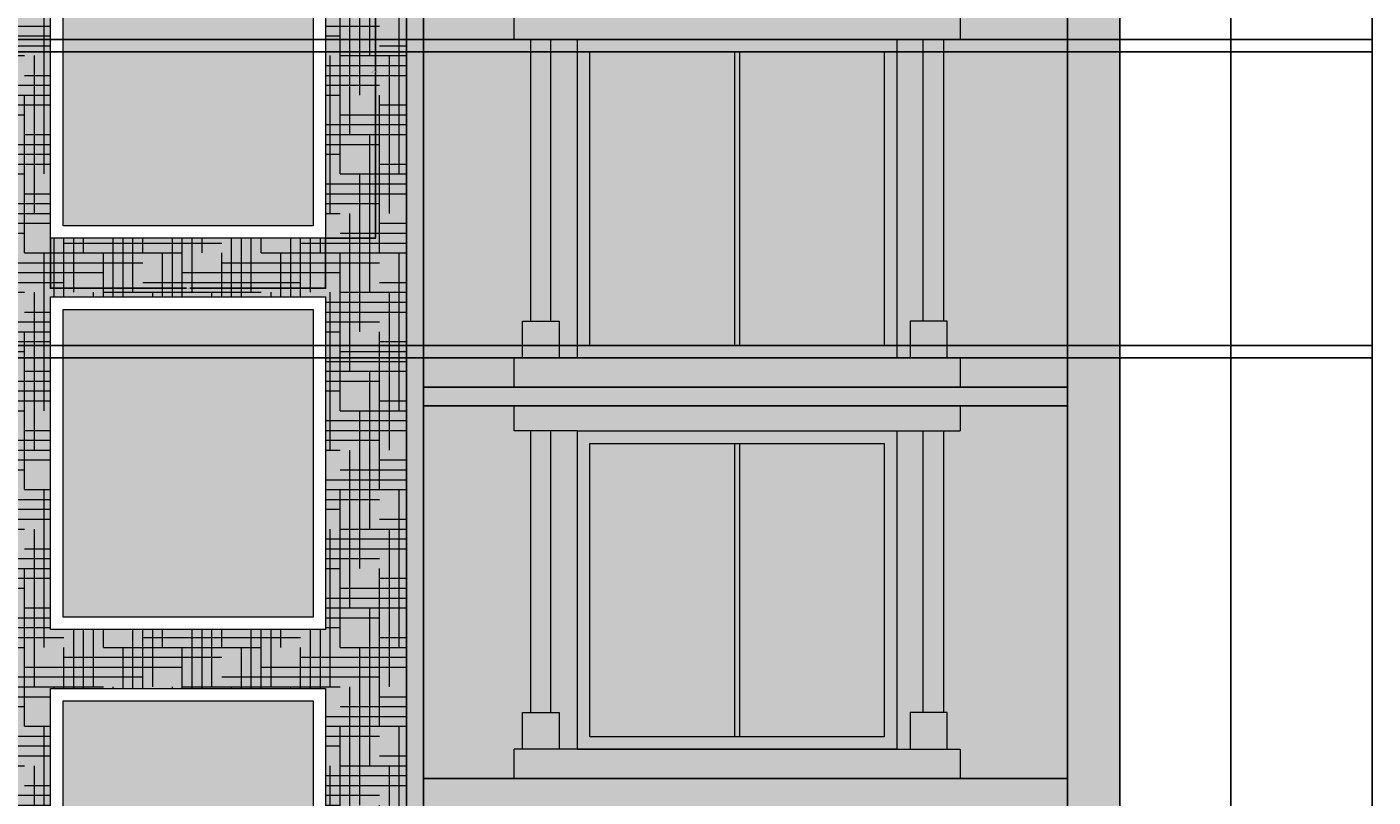
# Model space of a CAD drawing. Units: inches. Extents: x 3024 to 4744, y 1110 to 2100.
# Tile 26 of 29: x 3354 to 3787, y 1654 to 1902. Entities that reach past the tile are written whole.
import ezdxf

# ---------------------------------------------------------------- set-up
doc = ezdxf.new("R2010")
doc.units = ezdxf.units.IN
for name, color, linetype, lineweight in [('A-ANNO-DIMS', 2, 'Continuous', 18), ('A-ELEV', 7, 'Continuous', 25), ('A-ELEV-PATT', 252, 'Continuous', 13), ('A-GLAZ', 4, 'Continuous', 18)]:
    doc.layers.add(name, color=color, linetype=linetype, lineweight=lineweight)
doc.styles.get("Standard").update_dxf_attribs({"font": 'arial.ttf'})
doc.dimstyles.get("Standard").update_dxf_attribs({"dimtxt": 0.18, "dimasz": 0.18, "dimexe": 0.18, "dimexo": 0.0625, "dimgap": 0.09, "dimtad": 0, "dimtih": 1, "dimtoh": 1, "dimdec": 1, "dimzin": 0, "dimdsep": 46, "dimlunit": 3, "dimtxsty": 'Standard', "dimcen": 0.09, "dimadec": 0, "dimazin": 0, "dimtfac": 1, "dimtdec": 1, "dimtofl": 0, "dimtmove": 0, "dimatfit": 3, "dimfxl": 1, "dimtolj": 1, "dimtzin": 0, "dimarcsym": 0})

# ---------------------------------------------------------------- blocks, each defined once
blk = doc.blocks.new('WIN-BALCONY-A')
for p, q in [((3169.4, 1897.49), (3148.97, 1897.49)), ((3169.4, 1897.49), (3148.97, 1897.49)), ((3169.4, 1897.49), (3292.61, 1897.49)), ((3169.4, 1897.49), (3292.61, 1897.49)), ((3169.4, 1795.04), (3148.97, 1795.04)), ((3169.4, 1795.04), (3148.97, 1795.04)), ((3169.4, 1795.04), (3292.61, 1795.04)), ((3169.4, 1795.04), (3292.61, 1795.04))]:
    blk.add_line(p, q)
for points in [[(3148.97, 1897.49), (3148.97, 1905.61), (3292.61, 1905.61), (3292.61, 1897.49)], [(3148.97, 1897.49), (3148.97, 1905.61), (3292.61, 1905.61), (3292.61, 1897.49)], [(3292.61, 1795.04), (3292.61, 1785.61), (3148.97, 1785.61), (3148.97, 1795.04)], [(3292.61, 1795.04), (3292.61, 1785.61), (3148.97, 1785.61), (3148.97, 1795.04)]]:
    blk.add_lwpolyline(points)
for points in [[(3154.33, 1806.87), (3160.86, 1806.87), (3160.86, 1897.49), (3154.33, 1897.49)], [(3154.33, 1806.87), (3160.86, 1806.87), (3160.86, 1897.49), (3154.33, 1897.49)], [(3272.18, 1795.04), (3169.4, 1795.04), (3169.4, 1897.49), (3272.18, 1897.49)], [(3272.18, 1795.04), (3169.4, 1795.04), (3169.4, 1897.49), (3272.18, 1897.49)], [(3287.25, 1806.87), (3280.72, 1806.87), (3280.72, 1897.49), (3287.25, 1897.49)], [(3287.25, 1806.87), (3280.72, 1806.87), (3280.72, 1897.49), (3287.25, 1897.49)], [(3268.18, 1799.04), (3173.4, 1799.04), (3173.4, 1893.49), (3268.18, 1893.49)], [(3268.18, 1799.04), (3173.4, 1799.04), (3173.4, 1893.49), (3268.18, 1893.49)], [(3220.05, 1893.49), (3221.52, 1893.49), (3221.52, 1799.04), (3220.05, 1799.04)], [(3220.05, 1893.49), (3221.52, 1893.49), (3221.52, 1799.04), (3220.05, 1799.04)], [(3163.53, 1795.04), (3151.66, 1795.04), (3151.66, 1806.87), (3163.53, 1806.87)], [(3163.53, 1795.04), (3151.66, 1795.04), (3151.66, 1806.87), (3163.53, 1806.87)], [(3276.51, 1795.04), (3288.38, 1795.04), (3288.38, 1806.87), (3276.51, 1806.87)], [(3276.51, 1795.04), (3288.38, 1795.04), (3288.38, 1806.87), (3276.51, 1806.87)]]:
    blk.add_lwpolyline(points, close=True)
blk = doc.blocks.new('WIN-STONE-CENTRE')
for points in [[(3361.22, 1940.61), (3449.72, 1940.61), (3449.72, 1833.52), (3361.22, 1833.52)], [(3361.22, 1940.61), (3449.72, 1940.61), (3449.72, 1833.52), (3361.22, 1833.52)], [(3365.22, 1936.61), (3445.72, 1936.61), (3445.72, 1837.52), (3365.22, 1837.52)], [(3365.22, 1936.61), (3445.72, 1936.61), (3445.72, 1837.52), (3365.22, 1837.52)]]:
    blk.add_lwpolyline(points, close=True)
blk = doc.blocks.new('*D10')
at = {"layer": 'A-ANNO-DIMS', "color": 0, "lineweight": -2, "transparency": 16777216}
for p, q in [((3449.78, 1940.61), (3465.96, 1940.61)), ((3465.78, 1940.43), (3465.78, 1887.25)), ((3465.78, 1833.7), (3465.78, 1886.88)), ((3449.78, 1833.52), (3465.96, 1833.52))]:
    blk.add_line(p, q, dxfattribs=at)
at = {"layer": 'A-ANNO-DIMS', "color": 0, "transparency": 16777216}
for points in [[(3465.75, 1940.43), (3465.81, 1940.43), (3465.78, 1940.61)], [(3465.75, 1833.7), (3465.81, 1833.7), (3465.78, 1833.52)]]:
    blk.add_solid(points, dxfattribs=at)
at = {"layer": 'Defpoints', "color": 0, "transparency": 16777216}
for p in [(3449.72, 1940.61), (3465.78, 1940.61), (3449.72, 1833.52)]:
    blk.add_point(p, dxfattribs=at)
at = {"layer": 'A-ANNO-DIMS', "color": 0, "transparency": 16777216, "insert": (3465.78, 1887.07), "char_height": 0.18, "attachment_point": 5}
blk.add_mtext('\\A1;STONE WINDOW 107 TYP.', dxfattribs=at)
blk = doc.blocks.new('*D11')
at = {"layer": 'A-ANNO-DIMS', "color": 0, "lineweight": -2, "transparency": 16777216}
for p, q in [((3361.22, 1833.46), (3361.22, 1817.28)), ((3449.72, 1833.46), (3449.72, 1817.28)), ((3361.4, 1817.46), (3404.94, 1817.46)), ((3449.54, 1817.46), (3406, 1817.46))]:
    blk.add_line(p, q, dxfattribs=at)
at = {"layer": 'A-ANNO-DIMS', "color": 0, "transparency": 16777216}
for points in [[(3361.4, 1817.49), (3361.4, 1817.43), (3361.22, 1817.46)], [(3449.54, 1817.49), (3449.54, 1817.43), (3449.72, 1817.46)]]:
    blk.add_solid(points, dxfattribs=at)
at = {"layer": 'Defpoints', "color": 0, "transparency": 16777216}
for p in [(3361.22, 1833.52), (3449.72, 1833.52), (3449.72, 1817.46)]:
    blk.add_point(p, dxfattribs=at)
at = {"layer": 'A-ANNO-DIMS', "color": 0, "transparency": 16777216, "insert": (3405.47, 1817.46), "char_height": 0.18, "attachment_point": 5}
blk.add_mtext('\\A1;88 TYP.', dxfattribs=at)
blk = doc.blocks.new('*D64')
at = {"layer": 'A-ANNO-DIMS', "color": 0, "lineweight": -2, "transparency": 16777216}
for p, q in [((3069.79, 1241.5), (3069.79, 2100.44)), ((3069.97, 2100.26), (3405.08, 2100.26)), ((3740.97, 2100.26), (3405.87, 2100.26)), ((3741.15, 1241.5), (3741.15, 2100.44))]:
    blk.add_line(p, q, dxfattribs=at)
at = {"layer": 'A-ANNO-DIMS', "color": 0, "transparency": 16777216}
for points in [[(3069.97, 2100.29), (3069.97, 2100.23), (3069.79, 2100.26)], [(3740.97, 2100.29), (3740.97, 2100.23), (3741.15, 2100.26)]]:
    blk.add_solid(points, dxfattribs=at)
at = {"layer": 'Defpoints', "color": 0, "transparency": 16777216}
for p in [(3741.15, 2100.26), (3069.79, 1241.43), (3741.15, 1241.43)]:
    blk.add_point(p, dxfattribs=at)
at = {"layer": 'A-ANNO-DIMS', "color": 0, "transparency": 16777216, "insert": (3405.47, 2100.26), "char_height": 0.18, "attachment_point": 5}
blk.add_mtext('\\A1;671.4', dxfattribs=at)
blk = doc.blocks.new('*D75')
at = {"layer": 'A-ANNO-DIMS', "color": 0, "lineweight": -2, "transparency": 16777216}
for p, q in [((3491.89, 2054.76), (3786.83, 2054.76)), ((3786.65, 2054.58), (3786.65, 1605.37)), ((3786.65, 1155.79), (3786.65, 1605)), ((3741.21, 1155.61), (3786.83, 1155.61))]:
    blk.add_line(p, q, dxfattribs=at)
at = {"layer": 'A-ANNO-DIMS', "color": 0, "transparency": 16777216}
for points in [[(3786.62, 2054.58), (3786.68, 2054.58), (3786.65, 2054.76)], [(3786.62, 1155.79), (3786.68, 1155.79), (3786.65, 1155.61)]]:
    blk.add_solid(points, dxfattribs=at)
at = {"layer": 'Defpoints', "color": 0, "transparency": 16777216}
for p in [(3491.83, 2054.76), (3786.65, 2054.76), (3741.15, 1155.61)]:
    blk.add_point(p, dxfattribs=at)
at = {"layer": 'A-ANNO-DIMS', "color": 0, "transparency": 16777216, "insert": (3786.65, 1605.18), "char_height": 0.18, "attachment_point": 5}
blk.add_mtext('\\A1;899.1', dxfattribs=at)
blk = doc.blocks.new('*D100')
at = {"layer": 'A-ANNO-DIMS', "color": 0, "lineweight": -2, "transparency": 16777216}
for p, q in [((3268.24, 1799.04), (3786.83, 1799.04)), ((3786.65, 1798.86), (3786.65, 1797.23)), ((3272.24, 1795.04), (3786.83, 1795.04)), ((3786.65, 1795.22), (3786.65, 1796.86))]:
    blk.add_line(p, q, dxfattribs=at)
at = {"layer": 'A-ANNO-DIMS', "color": 0, "transparency": 16777216}
for points in [[(3786.62, 1798.86), (3786.68, 1798.86), (3786.65, 1799.04)], [(3786.62, 1795.22), (3786.68, 1795.22), (3786.65, 1795.04)]]:
    blk.add_solid(points, dxfattribs=at)
at = {"layer": 'Defpoints', "color": 0, "transparency": 16777216}
for p in [(3268.18, 1799.04), (3786.65, 1799.04), (3272.18, 1795.04)]:
    blk.add_point(p, dxfattribs=at)
at = {"layer": 'A-ANNO-DIMS', "color": 0, "transparency": 16777216, "insert": (3786.65, 1797.04), "char_height": 0.18, "attachment_point": 5}
blk.add_mtext('\\A1;4.00', dxfattribs=at)
blk = doc.blocks.new('*D101')
at = {"layer": 'A-ANNO-DIMS', "color": 0, "lineweight": -2, "transparency": 16777216}
for p, q in [((3268.24, 1893.49), (3786.83, 1893.49)), ((3786.65, 1893.31), (3786.65, 1846.45)), ((3786.65, 1799.22), (3786.65, 1846.08)), ((3268.24, 1799.04), (3786.83, 1799.04))]:
    blk.add_line(p, q, dxfattribs=at)
at = {"layer": 'A-ANNO-DIMS', "color": 0, "transparency": 16777216}
for points in [[(3786.62, 1893.31), (3786.68, 1893.31), (3786.65, 1893.49)], [(3786.62, 1799.22), (3786.68, 1799.22), (3786.65, 1799.04)]]:
    blk.add_solid(points, dxfattribs=at)
at = {"layer": 'Defpoints', "color": 0, "transparency": 16777216}
for p in [(3268.18, 1893.49), (3786.65, 1893.49), (3268.18, 1799.04)]:
    blk.add_point(p, dxfattribs=at)
at = {"layer": 'A-ANNO-DIMS', "color": 0, "transparency": 16777216, "insert": (3786.65, 1846.27), "char_height": 0.18, "attachment_point": 5}
blk.add_mtext('\\A1;94.44', dxfattribs=at)
blk = doc.blocks.new('*D102')
at = {"layer": 'A-ANNO-DIMS', "color": 0, "lineweight": -2, "transparency": 16777216}
for p, q in [((3272.24, 1897.49), (3786.83, 1897.49)), ((3786.65, 1897.31), (3786.65, 1895.67)), ((3786.65, 1893.67), (3786.65, 1895.31)), ((3268.24, 1893.49), (3786.83, 1893.49))]:
    blk.add_line(p, q, dxfattribs=at)
at = {"layer": 'A-ANNO-DIMS', "color": 0, "transparency": 16777216}
for points in [[(3786.62, 1897.31), (3786.68, 1897.31), (3786.65, 1897.49)], [(3786.62, 1893.67), (3786.68, 1893.67), (3786.65, 1893.49)]]:
    blk.add_solid(points, dxfattribs=at)
at = {"layer": 'Defpoints', "color": 0, "transparency": 16777216}
for p in [(3272.18, 1897.49), (3786.65, 1897.49), (3268.18, 1893.49)]:
    blk.add_point(p, dxfattribs=at)
at = {"layer": 'A-ANNO-DIMS', "color": 0, "transparency": 16777216, "insert": (3786.65, 1895.49), "char_height": 0.18, "attachment_point": 5}
blk.add_mtext('\\A1;4.00', dxfattribs=at)

msp = doc.modelspace()

# ---------------------------------------------------------------- hatches: boundary and pattern name
at = {"layer": 'A-ELEV-PATT'}
h = msp.add_hatch(color=256, dxfattribs=at)
h.dxf.hatch_style = 1
h.paths.add_polyline_path([(3491.8271, 2054.7584), (3320.5658, 2054.7584), (3320.5658, 2043.5286), (3491.8271, 2043.5286)])
h.paths.add_polyline_path([(3292.6051, 1905.6112), (3148.9694, 1905.6112), (3148.9694, 1897.4879), (3169.3964, 1897.4879), (3292.6051, 1897.4879)])
h.paths.add_polyline_path([(3292.6051, 1795.0431), (3169.3964, 1795.0431), (3148.9694, 1795.0431), (3148.9694, 1785.6112), (3292.6051, 1785.6112)])
h.paths.add_polyline_path([(3292.6051, 1779.6112), (3148.9694, 1779.6112), (3148.9694, 1771.4879), (3169.3964, 1771.4879), (3292.6051, 1771.4879)])
h.paths.add_polyline_path([(3292.6051, 1669.0431), (3169.3964, 1669.0431), (3148.9694, 1669.0431), (3148.9694, 1659.6112), (3292.6051, 1659.6112)])
h.paths.add_polyline_path([(3292.6051, 1653.6112), (3148.9694, 1653.6112), (3148.9694, 1645.4879), (3169.3964, 1645.4879), (3292.6051, 1645.4879)])
h.paths.add_polyline_path([(3292.6051, 1543.0431), (3169.3964, 1543.0431), (3148.9694, 1543.0431), (3148.9694, 1533.6112), (3292.6051, 1533.6112)])
h.paths.add_polyline_path([(3292.6051, 1527.6112), (3148.9694, 1527.6112), (3148.9694, 1519.4879), (3169.3964, 1519.4879), (3292.6051, 1519.4879)])
h.paths.add_polyline_path([(3292.6051, 1401.6112), (3148.9694, 1401.6112), (3148.9694, 1393.4879), (3169.3964, 1393.4879), (3292.6051, 1393.4879)])
h.paths.add_polyline_path([(3292.6051, 1417.0431), (3169.3964, 1417.0431), (3148.9694, 1417.0431), (3148.9694, 1407.6112), (3292.6051, 1407.6112)])
h.paths.add_polyline_path([(3292.6051, 1291.0431), (3169.3964, 1291.0431), (3148.9694, 1291.0431), (3148.9694, 1281.6112), (3292.6051, 1281.6112)])
h.paths.add_polyline_path([(3654.037, 1165.0431), (3530.8283, 1165.0431), (3510.4013, 1165.0431), (3510.4013, 1155.6112), (3654.037, 1155.6112)])
h.paths.add_polyline_path([(3654.037, 1275.6112), (3510.4013, 1275.6112), (3510.4013, 1267.4879), (3530.8283, 1267.4879), (3654.037, 1267.4879)])
h.paths.add_polyline_path([(3654.037, 1291.0431), (3530.8283, 1291.0431), (3510.4013, 1291.0431), (3510.4013, 1281.6112), (3654.037, 1281.6112)])
h.paths.add_polyline_path([(3654.037, 1417.0431), (3530.8283, 1417.0431), (3510.4013, 1417.0431), (3510.4013, 1407.6112), (3654.037, 1407.6112)])
h.paths.add_polyline_path([(3654.037, 1401.6112), (3510.4013, 1401.6112), (3510.4013, 1393.4879), (3530.8283, 1393.4879), (3654.037, 1393.4879)])
h.paths.add_polyline_path([(3654.037, 1543.0431), (3530.8283, 1543.0431), (3510.4013, 1543.0431), (3510.4013, 1533.6112), (3654.037, 1533.6112)])
h.paths.add_polyline_path([(3654.037, 1527.6112), (3510.4013, 1527.6112), (3510.4013, 1519.4879), (3530.8283, 1519.4879), (3654.037, 1519.4879)])
h.paths.add_polyline_path([(3654.037, 1653.6112), (3510.4013, 1653.6112), (3510.4013, 1645.4879), (3530.8283, 1645.4879), (3654.037, 1645.4879)])
h.paths.add_polyline_path([(3654.037, 1669.0431), (3530.8283, 1669.0431), (3510.4013, 1669.0431), (3510.4013, 1659.6112), (3654.037, 1659.6112)])
h.paths.add_polyline_path([(3654.037, 1779.6112), (3510.4013, 1779.6112), (3510.4013, 1771.4879), (3530.8283, 1771.4879), (3654.037, 1771.4879)])
h.paths.add_polyline_path([(3654.037, 1795.0431), (3530.8283, 1795.0431), (3510.4013, 1795.0431), (3510.4013, 1785.6112), (3654.037, 1785.6112)])
h.paths.add_polyline_path([(3654.037, 1905.6112), (3510.4013, 1905.6112), (3510.4013, 1897.4879), (3530.8283, 1897.4879), (3654.037, 1897.4879)])
h = msp.add_hatch(color=256, dxfattribs=at)
h.dxf.hatch_style = 1
h.paths.add_polyline_path([(3335.1044, 2043.5286), (3329.7033, 2043.5286), (3329.7033, 1155.6112), (3335.1044, 1155.6112)])
h.paths.add_polyline_path([(3481.2411, 2043.5286), (3335.1044, 2043.5286), (3335.1044, 1155.6112), (3481.2411, 1155.6112)])
h.paths.add_polyline_path([(3449.7202, 1329.5246), (3361.2242, 1329.5246), (3361.2242, 1436.6064), (3449.7202, 1436.6064)], flags=16)
h.paths.add_polyline_path([(3445.7202, 1333.5246), (3365.2242, 1333.5246), (3365.2242, 1432.6064), (3445.7202, 1432.6064)], flags=0)
h.paths.add_polyline_path([(3449.7202, 1455.5246), (3361.2242, 1455.5246), (3361.2242, 1562.6064), (3449.7202, 1562.6064)], flags=16)
h.paths.add_polyline_path([(3445.7202, 1459.5246), (3365.2242, 1459.5246), (3365.2242, 1558.6064), (3445.7202, 1558.6064)], flags=0)
h.paths.add_polyline_path([(3449.7202, 1581.5246), (3361.2242, 1581.5246), (3361.2242, 1688.6064), (3449.7202, 1688.6064)], flags=16)
h.paths.add_polyline_path([(3445.7202, 1585.5246), (3365.2242, 1585.5246), (3365.2242, 1684.6064), (3445.7202, 1684.6064)], flags=0)
h.paths.add_polyline_path([(3449.7202, 1707.5246), (3361.2242, 1707.5246), (3361.2242, 1814.6064), (3449.7202, 1814.6064)], flags=16)
h.paths.add_polyline_path([(3445.7202, 1711.5246), (3365.2242, 1711.5246), (3365.2242, 1810.6064), (3445.7202, 1810.6064)], flags=0)
h.paths.add_polyline_path([(3449.7202, 1833.5246), (3361.2242, 1833.5246), (3361.2242, 1940.6064), (3449.7202, 1940.6064)], flags=16)
h.paths.add_polyline_path([(3445.7202, 1837.5246), (3365.2242, 1837.5246), (3365.2242, 1936.6064), (3445.7202, 1936.6064)], flags=0)
h = msp.add_hatch(color=256, dxfattribs=at)
h.dxf.hatch_style = 1
h.paths.add_polyline_path([(3475.84, 2043.5286), (3335.1044, 2043.5286), (3335.1044, 1155.6112), (3475.84, 1155.6112)])
h.paths.add_polyline_path([(3449.7202, 1940.6064), (3449.7202, 1833.5246), (3361.2242, 1833.5246), (3361.2242, 1940.6064)], flags=16)
h.paths.add_polyline_path([(3445.7202, 1936.6064), (3445.7202, 1837.5246), (3365.2242, 1837.5246), (3365.2242, 1936.6064)], flags=0)
h.paths.add_polyline_path([(3449.7202, 1814.6064), (3449.7202, 1707.5246), (3361.2242, 1707.5246), (3361.2242, 1814.6064)], flags=16)
h.paths.add_polyline_path([(3445.7202, 1810.6064), (3445.7202, 1711.5246), (3365.2242, 1711.5246), (3365.2242, 1810.6064)], flags=0)
h.paths.add_polyline_path([(3449.7202, 1688.6064), (3449.7202, 1581.5246), (3361.2242, 1581.5246), (3361.2242, 1688.6064)], flags=16)
h.paths.add_polyline_path([(3445.7202, 1684.6064), (3445.7202, 1585.5246), (3365.2242, 1585.5246), (3365.2242, 1684.6064)], flags=0)
h.paths.add_polyline_path([(3449.7202, 1562.6064), (3449.7202, 1455.5246), (3361.2242, 1455.5246), (3361.2242, 1562.6064)], flags=16)
h.paths.add_polyline_path([(3445.7202, 1558.6064), (3445.7202, 1459.5246), (3365.2242, 1459.5246), (3365.2242, 1558.6064)], flags=0)
h.paths.add_polyline_path([(3449.7202, 1436.6064), (3449.7202, 1329.5246), (3361.2242, 1329.5246), (3361.2242, 1436.6064)], flags=16)
h.paths.add_polyline_path([(3445.7202, 1432.6064), (3445.7202, 1333.5246), (3365.2242, 1333.5246), (3365.2242, 1432.6064)], flags=0)
h = msp.add_hatch(dxfattribs=at)
h.set_pattern_fill('HOUND', color=256, scale=2)
h.paths.add_polyline_path([(3475.84, 2043.5286), (3335.1044, 2043.5286), (3335.1044, 1155.6112), (3475.84, 1155.6112)])
h.paths.add_polyline_path([(3449.7202, 1940.6064), (3449.7202, 1833.5246), (3361.2242, 1833.5246), (3361.2242, 1940.6064)], flags=16)
h.paths.add_polyline_path([(3445.7202, 1936.6064), (3445.7202, 1837.5246), (3365.2242, 1837.5246), (3365.2242, 1936.6064)], flags=0)
h.paths.add_polyline_path([(3449.7202, 1814.6064), (3449.7202, 1707.5246), (3361.2242, 1707.5246), (3361.2242, 1814.6064)], flags=16)
h.paths.add_polyline_path([(3445.7202, 1810.6064), (3445.7202, 1711.5246), (3365.2242, 1711.5246), (3365.2242, 1810.6064)], flags=0)
h.paths.add_polyline_path([(3449.7202, 1688.6064), (3449.7202, 1581.5246), (3361.2242, 1581.5246), (3361.2242, 1688.6064)], flags=16)
h.paths.add_polyline_path([(3445.7202, 1684.6064), (3445.7202, 1585.5246), (3365.2242, 1585.5246), (3365.2242, 1684.6064)], flags=0)
h.paths.add_polyline_path([(3449.7202, 1562.6064), (3449.7202, 1455.5246), (3361.2242, 1455.5246), (3361.2242, 1562.6064)], flags=16)
h.paths.add_polyline_path([(3445.7202, 1558.6064), (3445.7202, 1459.5246), (3365.2242, 1459.5246), (3365.2242, 1558.6064)], flags=0)
h.paths.add_polyline_path([(3449.7202, 1436.6064), (3449.7202, 1329.5246), (3361.2242, 1329.5246), (3361.2242, 1436.6064)], flags=16)
h.paths.add_polyline_path([(3445.7202, 1432.6064), (3445.7202, 1333.5246), (3365.2242, 1333.5246), (3365.2242, 1432.6064)], flags=0)
h = msp.add_hatch(color=256, dxfattribs=at)
h.dxf.hatch_style = 1
h.paths.add_polyline_path([(3582.956, 2019.4879), (3581.4824, 2019.4879), (3581.4824, 1925.0431), (3582.956, 1925.0431)], flags=0)
h.paths.add_polyline_path([(3582.956, 2019.4879), (3582.956, 1925.0431), (3581.4824, 1925.0431), (3581.4824, 2019.4879)], flags=0)
h.paths.add_polyline_path([(3582.956, 1893.4879), (3581.4824, 1893.4879), (3581.4824, 1799.0431), (3582.956, 1799.0431)])
h = msp.add_hatch(color=256, dxfattribs=at)
h.dxf.hatch_style = 1
h.paths.add_polyline_path([(3705.4722, 2014.6567), (3688.5588, 2014.6567), (3481.2411, 2014.6567), (3481.2411, 2009.1664), (3688.5588, 2009.1664), (3688.5588, 1155.6112), (3705.4722, 1155.6112), (3705.4722, 1911.6112)])
h = msp.add_hatch(color=256, dxfattribs=at)
h.dxf.hatch_style = 1
h.paths.add_polyline_path([(3445.7202, 1936.6064), (3365.2242, 1936.6064), (3365.2242, 1837.5246), (3445.7202, 1837.5246)])
h.paths.add_polyline_path([(3445.7202, 1810.6064), (3365.2242, 1810.6064), (3365.2242, 1711.5246), (3445.7202, 1711.5246)])
h.paths.add_polyline_path([(3445.7202, 1684.6064), (3365.2242, 1684.6064), (3365.2242, 1585.5246), (3445.7202, 1585.5246)])
h.paths.add_polyline_path([(3445.7202, 1558.6064), (3365.2242, 1558.6064), (3365.2242, 1459.5246), (3445.7202, 1459.5246)])
h.paths.add_polyline_path([(3445.7202, 1432.6064), (3365.2242, 1432.6064), (3365.2242, 1333.5246), (3445.7202, 1333.5246)])
h = msp.add_hatch(color=256, dxfattribs=at)
h.dxf.hatch_style = 1
h.paths.add_polyline_path([(3154.3287, 1897.4879), (3148.9694, 1897.4879), (3148.9694, 1905.6112), (3105.4722, 1905.6112), (3105.4722, 1785.6112), (3148.9694, 1785.6112), (3148.9694, 1795.0431), (3151.6604, 1795.0431), (3151.6604, 1806.8674), (3154.3287, 1806.8674)])
h.paths.add_polyline_path([(3329.7033, 1905.6112), (3292.6051, 1905.6112), (3292.6051, 1897.4879), (3287.2458, 1897.4879), (3287.2458, 1806.8674), (3288.3759, 1806.8674), (3288.3759, 1795.0431), (3292.6051, 1795.0431), (3292.6051, 1785.6112), (3329.7033, 1785.6112)])
h.paths.add_polyline_path([(3154.3287, 1771.4879), (3148.9694, 1771.4879), (3148.9694, 1779.6112), (3105.4722, 1779.6112), (3105.4722, 1659.6112), (3148.9694, 1659.6112), (3148.9694, 1669.0431), (3151.6604, 1669.0431), (3151.6604, 1680.8674), (3154.3287, 1680.8674)])
h.paths.add_polyline_path([(3329.7033, 1779.6112), (3292.6051, 1779.6112), (3292.6051, 1771.4879), (3287.2458, 1771.4879), (3287.2458, 1680.8674), (3288.3759, 1680.8674), (3288.3759, 1669.0431), (3292.6051, 1669.0431), (3292.6051, 1659.6112), (3329.7033, 1659.6112)])
h.paths.add_polyline_path([(3154.3287, 1645.4879), (3148.9694, 1645.4879), (3148.9694, 1653.6112), (3105.4722, 1653.6112), (3105.4722, 1533.6112), (3148.9694, 1533.6112), (3148.9694, 1543.0431), (3151.6604, 1543.0431), (3151.6604, 1554.8674), (3154.3287, 1554.8674)])
h.paths.add_polyline_path([(3329.7033, 1653.6112), (3292.6051, 1653.6112), (3292.6051, 1645.4879), (3287.2458, 1645.4879), (3287.2458, 1554.8674), (3288.3759, 1554.8674), (3288.3759, 1543.0431), (3292.6051, 1543.0431), (3292.6051, 1533.6112), (3329.7033, 1533.6112)])
h.paths.add_polyline_path([(3329.7033, 1527.6112), (3292.6051, 1527.6112), (3292.6051, 1519.4879), (3287.2458, 1519.4879), (3287.2458, 1428.8674), (3288.3759, 1428.8674), (3288.3759, 1417.0431), (3292.6051, 1417.0431), (3292.6051, 1407.6112), (3329.7033, 1407.6112)])
h.paths.add_polyline_path([(3329.7033, 1401.6112), (3292.6051, 1401.6112), (3292.6051, 1393.4879), (3287.2458, 1393.4879), (3287.2458, 1302.8674), (3288.3759, 1302.8674), (3288.3759, 1291.0431), (3292.6051, 1291.0431), (3292.6051, 1281.6112), (3329.7033, 1281.6112)])
h.paths.add_polyline_path([(3154.3287, 1393.4879), (3148.9694, 1393.4879), (3148.9694, 1401.6112), (3105.4722, 1401.6112), (3105.4722, 1281.6112), (3148.9694, 1281.6112), (3148.9694, 1291.0431), (3151.6604, 1291.0431), (3151.6604, 1302.8674), (3154.3287, 1302.8674)])
h.paths.add_polyline_path([(3154.3287, 1519.4879), (3148.9694, 1519.4879), (3148.9694, 1527.6112), (3105.4722, 1527.6112), (3105.4722, 1407.6112), (3148.9694, 1407.6112), (3148.9694, 1417.0431), (3151.6604, 1417.0431), (3151.6604, 1428.8674), (3154.3287, 1428.8674)])
h.paths.add_polyline_path([(3515.7606, 1897.4879), (3510.4013, 1897.4879), (3510.4013, 1905.6112), (3481.2411, 1905.6112), (3481.2411, 1785.6112), (3510.4013, 1785.6112), (3510.4013, 1795.0431), (3513.0923, 1795.0431), (3513.0923, 1806.8674), (3515.7606, 1806.8674)])
h.paths.add_polyline_path([(3688.5588, 1905.6112), (3654.037, 1905.6112), (3654.037, 1897.4879), (3648.6777, 1897.4879), (3648.6777, 1806.8674), (3649.8078, 1806.8674), (3649.8078, 1795.0431), (3654.037, 1795.0431), (3654.037, 1785.6112), (3688.5588, 1785.6112)])
h.paths.add_polyline_path([(3515.7606, 1771.4879), (3510.4013, 1771.4879), (3510.4013, 1779.6112), (3481.2411, 1779.6112), (3481.2411, 1659.6112), (3510.4013, 1659.6112), (3510.4013, 1669.0431), (3513.0923, 1669.0431), (3513.0923, 1680.8674), (3515.7606, 1680.8674)])
h.paths.add_polyline_path([(3688.5588, 1779.6112), (3654.037, 1779.6112), (3654.037, 1771.4879), (3648.6777, 1771.4879), (3648.6777, 1680.8674), (3649.8078, 1680.8674), (3649.8078, 1669.0431), (3654.037, 1669.0431), (3654.037, 1659.6112), (3688.5588, 1659.6112)])
h.paths.add_polyline_path([(3515.7606, 1645.4879), (3510.4013, 1645.4879), (3510.4013, 1653.6112), (3481.2411, 1653.6112), (3481.2411, 1533.6112), (3510.4013, 1533.6112), (3510.4013, 1543.0431), (3513.0923, 1543.0431), (3513.0923, 1554.8674), (3515.7606, 1554.8674)])
h.paths.add_polyline_path([(3688.5588, 1653.6112), (3654.037, 1653.6112), (3654.037, 1645.4879), (3648.6777, 1645.4879), (3648.6777, 1554.8674), (3649.8078, 1554.8674), (3649.8078, 1543.0431), (3654.037, 1543.0431), (3654.037, 1533.6112), (3688.5588, 1533.6112)])
h.paths.add_polyline_path([(3515.7606, 1519.4879), (3510.4013, 1519.4879), (3510.4013, 1527.6112), (3481.2411, 1527.6112), (3481.2411, 1407.6112), (3510.4013, 1407.6112), (3510.4013, 1417.0431), (3513.0923, 1417.0431), (3513.0923, 1428.8674), (3515.7606, 1428.8674)])
h.paths.add_polyline_path([(3688.5588, 1527.6112), (3654.037, 1527.6112), (3654.037, 1519.4879), (3648.6777, 1519.4879), (3648.6777, 1428.8674), (3649.8078, 1428.8674), (3649.8078, 1417.0431), (3654.037, 1417.0431), (3654.037, 1407.6112), (3688.5588, 1407.6112)])
h.paths.add_polyline_path([(3515.7606, 1393.4879), (3510.4013, 1393.4879), (3510.4013, 1401.6112), (3481.2411, 1401.6112), (3481.2411, 1281.6112), (3510.4013, 1281.6112), (3510.4013, 1291.0431), (3513.0923, 1291.0431), (3513.0923, 1302.8674), (3515.7606, 1302.8674)])
h.paths.add_polyline_path([(3688.5588, 1401.6112), (3654.037, 1401.6112), (3654.037, 1393.4879), (3648.6777, 1393.4879), (3648.6777, 1302.8674), (3649.8078, 1302.8674), (3649.8078, 1291.0431), (3654.037, 1291.0431), (3654.037, 1281.6112), (3688.5588, 1281.6112)])
h.paths.add_polyline_path([(3515.7606, 1267.4879), (3510.4013, 1267.4879), (3510.4013, 1275.6112), (3481.2411, 1275.6112), (3481.2411, 1155.6112), (3510.4013, 1155.6112), (3510.4013, 1165.0431), (3513.0923, 1165.0431), (3513.0923, 1176.8674), (3515.7606, 1176.8674)])
h.paths.add_polyline_path([(3688.5588, 1275.6112), (3654.037, 1275.6112), (3654.037, 1267.4879), (3648.6777, 1267.4879), (3648.6777, 1176.8674), (3649.8078, 1176.8674), (3649.8078, 1165.0431), (3654.037, 1165.0431), (3654.037, 1155.6112), (3688.5588, 1155.6112)])
h.paths.add_polyline_path([(3112.3838, 1275.6112), (3105.4722, 1275.6112), (3105.4722, 1171.0239), (3112.3838, 1171.0239)])
h = msp.add_hatch(color=256, dxfattribs=at)
h.dxf.hatch_style = 1
h.paths.add_polyline_path([(3160.8586, 1897.4879), (3154.3287, 1897.4879), (3154.3287, 1806.8674), (3160.8586, 1806.8674)])
h.paths.add_polyline_path([(3287.2458, 1897.4879), (3280.716, 1897.4879), (3280.716, 1806.8674), (3287.2458, 1806.8674)])
h.paths.add_polyline_path([(3160.8586, 1771.4879), (3154.3287, 1771.4879), (3154.3287, 1680.8674), (3160.8586, 1680.8674)])
h.paths.add_polyline_path([(3287.2458, 1771.4879), (3280.716, 1771.4879), (3280.716, 1680.8674), (3287.2458, 1680.8674)])
h.paths.add_polyline_path([(3160.8586, 1645.4879), (3154.3287, 1645.4879), (3154.3287, 1554.8674), (3160.8586, 1554.8674)])
h.paths.add_polyline_path([(3287.2458, 1645.4879), (3280.716, 1645.4879), (3280.716, 1554.8674), (3287.2458, 1554.8674)])
h.paths.add_polyline_path([(3160.8586, 1519.4879), (3154.3287, 1519.4879), (3154.3287, 1428.8674), (3160.8586, 1428.8674)])
h.paths.add_polyline_path([(3287.2458, 1519.4879), (3280.716, 1519.4879), (3280.716, 1428.8674), (3287.2458, 1428.8674)])
h.paths.add_polyline_path([(3160.8586, 1393.4879), (3154.3287, 1393.4879), (3154.3287, 1302.8674), (3160.8586, 1302.8674)])
h.paths.add_polyline_path([(3287.2458, 1393.4879), (3280.716, 1393.4879), (3280.716, 1302.8674), (3287.2458, 1302.8674)])
h.paths.add_polyline_path([(3648.6777, 1267.4879), (3642.1479, 1267.4879), (3642.1479, 1176.8674), (3648.6777, 1176.8674)])
h.paths.add_polyline_path([(3522.2905, 1267.4879), (3515.7606, 1267.4879), (3515.7606, 1176.8674), (3522.2905, 1176.8674)])
h.paths.add_polyline_path([(3522.2905, 1393.4879), (3515.7606, 1393.4879), (3515.7606, 1302.8674), (3522.2905, 1302.8674)])
h.paths.add_polyline_path([(3648.6777, 1393.4879), (3642.1479, 1393.4879), (3642.1479, 1302.8674), (3648.6777, 1302.8674)])
h.paths.add_polyline_path([(3522.2905, 1519.4879), (3515.7606, 1519.4879), (3515.7606, 1428.8674), (3522.2905, 1428.8674)])
h.paths.add_polyline_path([(3648.6777, 1519.4879), (3642.1479, 1519.4879), (3642.1479, 1428.8674), (3648.6777, 1428.8674)])
h.paths.add_polyline_path([(3522.2905, 1645.4879), (3515.7606, 1645.4879), (3515.7606, 1554.8674), (3522.2905, 1554.8674)])
h.paths.add_polyline_path([(3522.2905, 1771.4879), (3515.7606, 1771.4879), (3515.7606, 1680.8674), (3522.2905, 1680.8674)])
h.paths.add_polyline_path([(3648.6777, 1645.4879), (3642.1479, 1645.4879), (3642.1479, 1554.8674), (3648.6777, 1554.8674)])
h.paths.add_polyline_path([(3648.6777, 1771.4879), (3642.1479, 1771.4879), (3642.1479, 1680.8674), (3648.6777, 1680.8674)])
h.paths.add_polyline_path([(3648.6777, 1897.4879), (3642.1479, 1897.4879), (3642.1479, 1806.8674), (3648.6777, 1806.8674)])
h.paths.add_polyline_path([(3522.2905, 1897.4879), (3515.7606, 1897.4879), (3515.7606, 1806.8674), (3522.2905, 1806.8674)])
h = msp.add_hatch(color=256, dxfattribs=at)
h.dxf.hatch_style = 1
h.paths.add_polyline_path([(3169.3964, 1897.4879), (3160.8586, 1897.4879), (3160.8586, 1806.8674), (3163.5269, 1806.8674), (3163.5269, 1795.0431), (3169.3964, 1795.0431)])
h.paths.add_polyline_path([(3280.716, 1897.4879), (3272.1781, 1897.4879), (3272.1781, 1795.0431), (3276.5094, 1795.0431), (3276.5094, 1806.8674), (3280.716, 1806.8674)])
h.paths.add_polyline_path([(3280.716, 1771.4879), (3272.1781, 1771.4879), (3272.1781, 1669.0431), (3276.5094, 1669.0431), (3276.5094, 1680.8674), (3280.716, 1680.8674)])
h.paths.add_polyline_path([(3169.3964, 1771.4879), (3160.8586, 1771.4879), (3160.8586, 1680.8674), (3163.5269, 1680.8674), (3163.5269, 1669.0431), (3169.3964, 1669.0431)])
h.paths.add_polyline_path([(3169.3964, 1645.4879), (3160.8586, 1645.4879), (3160.8586, 1554.8674), (3163.5269, 1554.8674), (3163.5269, 1543.0431), (3169.3964, 1543.0431)])
h.paths.add_polyline_path([(3280.716, 1645.4879), (3272.1781, 1645.4879), (3272.1781, 1543.0431), (3276.5094, 1543.0431), (3276.5094, 1554.8674), (3280.716, 1554.8674)])
h.paths.add_polyline_path([(3169.3964, 1519.4879), (3160.8586, 1519.4879), (3160.8586, 1428.8674), (3163.5269, 1428.8674), (3163.5269, 1417.0431), (3169.3964, 1417.0431)])
h.paths.add_polyline_path([(3280.716, 1519.4879), (3272.1781, 1519.4879), (3272.1781, 1417.0431), (3276.5094, 1417.0431), (3276.5094, 1428.8674), (3280.716, 1428.8674)])
h.paths.add_polyline_path([(3169.3964, 1393.4879), (3160.8586, 1393.4879), (3160.8586, 1302.8674), (3163.5269, 1302.8674), (3163.5269, 1291.0431), (3169.3964, 1291.0431)])
h.paths.add_polyline_path([(3280.716, 1393.4879), (3272.1781, 1393.4879), (3272.1781, 1291.0431), (3276.5094, 1291.0431), (3276.5094, 1302.8674), (3280.716, 1302.8674)])
h.paths.add_polyline_path([(3642.1479, 1267.4879), (3633.61, 1267.4879), (3633.61, 1165.0431), (3637.9413, 1165.0431), (3637.9413, 1176.8674), (3642.1479, 1176.8674)])
h.paths.add_polyline_path([(3530.8283, 1267.4879), (3522.2905, 1267.4879), (3522.2905, 1176.8674), (3524.9588, 1176.8674), (3524.9588, 1165.0431), (3530.8283, 1165.0431)])
h.paths.add_polyline_path([(3642.1479, 1393.4879), (3633.61, 1393.4879), (3633.61, 1291.0431), (3637.9413, 1291.0431), (3637.9413, 1302.8674), (3642.1479, 1302.8674)])
h.paths.add_polyline_path([(3530.8283, 1393.4879), (3522.2905, 1393.4879), (3522.2905, 1302.8674), (3524.9588, 1302.8674), (3524.9588, 1291.0431), (3530.8283, 1291.0431)])
h.paths.add_polyline_path([(3530.8283, 1519.4879), (3522.2905, 1519.4879), (3522.2905, 1428.8674), (3524.9588, 1428.8674), (3524.9588, 1417.0431), (3530.8283, 1417.0431)])
h.paths.add_polyline_path([(3642.1479, 1519.4879), (3633.61, 1519.4879), (3633.61, 1417.0431), (3637.9413, 1417.0431), (3637.9413, 1428.8674), (3642.1479, 1428.8674)])
h.paths.add_polyline_path([(3530.8283, 1645.4879), (3522.2905, 1645.4879), (3522.2905, 1554.8674), (3524.9588, 1554.8674), (3524.9588, 1543.0431), (3530.8283, 1543.0431)])
h.paths.add_polyline_path([(3642.1479, 1645.4879), (3633.61, 1645.4879), (3633.61, 1543.0431), (3637.9413, 1543.0431), (3637.9413, 1554.8674), (3642.1479, 1554.8674)])
h.paths.add_polyline_path([(3642.1479, 1771.4879), (3633.61, 1771.4879), (3633.61, 1669.0431), (3637.9413, 1669.0431), (3637.9413, 1680.8674), (3642.1479, 1680.8674)])
h.paths.add_polyline_path([(3530.8283, 1771.4879), (3522.2905, 1771.4879), (3522.2905, 1680.8674), (3524.9588, 1680.8674), (3524.9588, 1669.0431), (3530.8283, 1669.0431)])
h.paths.add_polyline_path([(3530.8283, 1897.4879), (3522.2905, 1897.4879), (3522.2905, 1806.8674), (3524.9588, 1806.8674), (3524.9588, 1795.0431), (3530.8283, 1795.0431)])
h.paths.add_polyline_path([(3642.1479, 1897.4879), (3633.61, 1897.4879), (3633.61, 1795.0431), (3637.9413, 1795.0431), (3637.9413, 1806.8674), (3642.1479, 1806.8674)])
h = msp.add_hatch(color=256, dxfattribs=at)
h.dxf.hatch_style = 1
h.paths.add_polyline_path([(3582.956, 1893.4879), (3581.4824, 1893.4879), (3581.4824, 1799.0431), (3582.956, 1799.0431)], flags=0)
h.paths.add_polyline_path([(3633.61, 1897.4879), (3530.8283, 1897.4879), (3530.8283, 1795.0431), (3633.61, 1795.0431)])
h.paths.add_polyline_path([(3629.61, 1893.4879), (3629.61, 1799.0431), (3534.8283, 1799.0431), (3534.8283, 1893.4879)], flags=16)
h.paths.add_polyline_path([(3582.956, 1893.4879), (3582.956, 1799.0431), (3581.4824, 1799.0431), (3581.4824, 1893.4879)], flags=0)
h = msp.add_hatch(color=256, dxfattribs=at)
h.dxf.hatch_style = 1
h.paths.add_polyline_path([(3220.0505, 1893.4879), (3173.3964, 1893.4879), (3173.3964, 1799.0431), (3220.0505, 1799.0431)])
h.paths.add_polyline_path([(3268.1781, 1893.4879), (3221.5241, 1893.4879), (3221.5241, 1799.0431), (3268.1781, 1799.0431)])
h.paths.add_polyline_path([(3581.4824, 1893.4879), (3534.8283, 1893.4879), (3534.8283, 1799.0431), (3581.4824, 1799.0431)])
h.paths.add_polyline_path([(3629.61, 1893.4879), (3582.956, 1893.4879), (3582.956, 1799.0431), (3629.61, 1799.0431)])
h.paths.add_polyline_path([(3581.4824, 1767.4879), (3534.8283, 1767.4879), (3534.8283, 1673.0431), (3581.4824, 1673.0431)])
h.paths.add_polyline_path([(3629.61, 1767.4879), (3582.956, 1767.4879), (3582.956, 1673.0431), (3629.61, 1673.0431)])
h.paths.add_polyline_path([(3581.4824, 1641.4879), (3534.8283, 1641.4879), (3534.8283, 1547.0431), (3581.4824, 1547.0431)])
h.paths.add_polyline_path([(3629.61, 1641.4879), (3582.956, 1641.4879), (3582.956, 1547.0431), (3629.61, 1547.0431)])
h.paths.add_polyline_path([(3629.61, 1515.4879), (3582.956, 1515.4879), (3582.956, 1421.0431), (3629.61, 1421.0431)])
h.paths.add_polyline_path([(3581.4824, 1515.4879), (3534.8283, 1515.4879), (3534.8283, 1421.0431), (3581.4824, 1421.0431)])
h.paths.add_polyline_path([(3629.61, 1389.4879), (3582.956, 1389.4879), (3582.956, 1295.0431), (3629.61, 1295.0431)])
h.paths.add_polyline_path([(3581.4824, 1389.4879), (3534.8283, 1389.4879), (3534.8283, 1295.0431), (3581.4824, 1295.0431)])
h.paths.add_polyline_path([(3629.61, 1263.4879), (3582.956, 1263.4879), (3582.956, 1169.0431), (3629.61, 1169.0431)])
h.paths.add_polyline_path([(3581.4824, 1263.4879), (3534.8283, 1263.4879), (3534.8283, 1169.0431), (3581.4824, 1169.0431)])
h.paths.add_polyline_path([(3220.0505, 1389.4879), (3173.3964, 1389.4879), (3173.3964, 1295.0431), (3220.0505, 1295.0431)])
h.paths.add_polyline_path([(3268.1781, 1389.4879), (3221.5241, 1389.4879), (3221.5241, 1295.0431), (3268.1781, 1295.0431)])
h.paths.add_polyline_path([(3220.0505, 1515.4879), (3173.3964, 1515.4879), (3173.3964, 1421.0431), (3220.0505, 1421.0431)])
h.paths.add_polyline_path([(3268.1781, 1515.4879), (3221.5241, 1515.4879), (3221.5241, 1421.0431), (3268.1781, 1421.0431)])
h.paths.add_polyline_path([(3220.0505, 1767.4879), (3173.3964, 1767.4879), (3173.3964, 1673.0431), (3220.0505, 1673.0431)])
h.paths.add_polyline_path([(3268.1781, 1767.4879), (3221.5241, 1767.4879), (3221.5241, 1673.0431), (3268.1781, 1673.0431)])
h.paths.add_polyline_path([(3220.0505, 1641.4879), (3173.3964, 1641.4879), (3173.3964, 1547.0431), (3220.0505, 1547.0431)])
h.paths.add_polyline_path([(3268.1781, 1641.4879), (3221.5241, 1641.4879), (3221.5241, 1547.0431), (3268.1781, 1547.0431)])
h = msp.add_hatch(color=256, dxfattribs=at)
h.dxf.hatch_style = 1
h.paths.add_polyline_path([(3582.956, 1893.4879), (3581.4824, 1893.4879), (3581.4824, 1799.0431), (3582.956, 1799.0431)], flags=0)
h.paths.add_polyline_path([(3582.956, 1893.4879), (3582.956, 1799.0431), (3581.4824, 1799.0431), (3581.4824, 1893.4879)], flags=0)
h.paths.add_polyline_path([(3582.956, 1767.4879), (3581.4824, 1767.4879), (3581.4824, 1673.0431), (3582.956, 1673.0431)])
h = msp.add_hatch(color=256, dxfattribs=at)
h.dxf.hatch_style = 1
h.paths.add_polyline_path([(3163.5269, 1302.8674), (3151.6604, 1302.8674), (3151.6604, 1291.0431), (3163.5269, 1291.0431)])
h.paths.add_polyline_path([(3288.3759, 1302.8674), (3276.5094, 1302.8674), (3276.5094, 1291.0431), (3288.3759, 1291.0431)])
h.paths.add_polyline_path([(3288.3759, 1428.8674), (3276.5094, 1428.8674), (3276.5094, 1417.0431), (3288.3759, 1417.0431)])
h.paths.add_polyline_path([(3163.5269, 1428.8674), (3151.6604, 1428.8674), (3151.6604, 1417.0431), (3163.5269, 1417.0431)])
h.paths.add_polyline_path([(3163.5269, 1554.8674), (3151.6604, 1554.8674), (3151.6604, 1543.0431), (3163.5269, 1543.0431)])
h.paths.add_polyline_path([(3288.3759, 1554.8674), (3276.5094, 1554.8674), (3276.5094, 1543.0431), (3288.3759, 1543.0431)])
h.paths.add_polyline_path([(3163.5269, 1680.8674), (3151.6604, 1680.8674), (3151.6604, 1669.0431), (3163.5269, 1669.0431)])
h.paths.add_polyline_path([(3288.3759, 1680.8674), (3276.5094, 1680.8674), (3276.5094, 1669.0431), (3288.3759, 1669.0431)])
h.paths.add_polyline_path([(3163.5269, 1806.8674), (3151.6604, 1806.8674), (3151.6604, 1795.0431), (3163.5269, 1795.0431)])
h.paths.add_polyline_path([(3288.3759, 1806.8674), (3276.5094, 1806.8674), (3276.5094, 1795.0431), (3288.3759, 1795.0431)])
h.paths.add_polyline_path([(3524.9588, 1806.8674), (3513.0923, 1806.8674), (3513.0923, 1795.0431), (3524.9588, 1795.0431)])
h.paths.add_polyline_path([(3649.8078, 1806.8674), (3637.9413, 1806.8674), (3637.9413, 1795.0431), (3649.8078, 1795.0431)])
h.paths.add_polyline_path([(3524.9588, 1680.8674), (3513.0923, 1680.8674), (3513.0923, 1669.0431), (3524.9588, 1669.0431)])
h.paths.add_polyline_path([(3649.8078, 1680.8674), (3637.9413, 1680.8674), (3637.9413, 1669.0431), (3649.8078, 1669.0431)])
h.paths.add_polyline_path([(3524.9588, 1554.8674), (3513.0923, 1554.8674), (3513.0923, 1543.0431), (3524.9588, 1543.0431)])
h.paths.add_polyline_path([(3649.8078, 1554.8674), (3637.9413, 1554.8674), (3637.9413, 1543.0431), (3649.8078, 1543.0431)])
h.paths.add_polyline_path([(3524.9588, 1428.8674), (3513.0923, 1428.8674), (3513.0923, 1417.0431), (3524.9588, 1417.0431)])
h.paths.add_polyline_path([(3649.8078, 1428.8674), (3637.9413, 1428.8674), (3637.9413, 1417.0431), (3649.8078, 1417.0431)])
h.paths.add_polyline_path([(3524.9588, 1302.8674), (3513.0923, 1302.8674), (3513.0923, 1291.0431), (3524.9588, 1291.0431)])
h.paths.add_polyline_path([(3649.8078, 1302.8674), (3637.9413, 1302.8674), (3637.9413, 1291.0431), (3649.8078, 1291.0431)])
h.paths.add_polyline_path([(3524.9588, 1176.8674), (3513.0923, 1176.8674), (3513.0923, 1165.0431), (3524.9588, 1165.0431)])
h.paths.add_polyline_path([(3649.8078, 1176.8674), (3637.9413, 1176.8674), (3637.9413, 1165.0431), (3649.8078, 1165.0431)])
h = msp.add_hatch(color=256, dxfattribs=at)
h.dxf.hatch_style = 1
h.paths.add_polyline_path([(3688.5588, 1785.6112), (3481.2411, 1785.6112), (3481.2411, 1779.6112), (3688.5588, 1779.6112)])
h.paths.add_polyline_path([(3688.5588, 1659.6112), (3481.2411, 1659.6112), (3481.2411, 1653.6112), (3688.5588, 1653.6112)])
h.paths.add_polyline_path([(3688.5588, 1533.6112), (3481.2411, 1533.6112), (3481.2411, 1527.6112), (3688.5588, 1527.6112)])
h.paths.add_polyline_path([(3688.5588, 1407.6112), (3481.2411, 1407.6112), (3481.2411, 1401.6112), (3688.5588, 1401.6112)])
h.paths.add_polyline_path([(3688.5588, 1281.6112), (3481.2411, 1281.6112), (3481.2411, 1275.6112), (3688.5588, 1275.6112)])
h = msp.add_hatch(color=256, dxfattribs=at)
h.dxf.hatch_style = 1
h.paths.add_polyline_path([(3582.956, 1767.4879), (3581.4824, 1767.4879), (3581.4824, 1673.0431), (3582.956, 1673.0431)], flags=0)
h.paths.add_polyline_path([(3633.61, 1771.4879), (3530.8283, 1771.4879), (3530.8283, 1669.0431), (3633.61, 1669.0431)])
h.paths.add_polyline_path([(3629.61, 1767.4879), (3629.61, 1673.0431), (3534.8283, 1673.0431), (3534.8283, 1767.4879)], flags=16)
h.paths.add_polyline_path([(3582.956, 1767.4879), (3582.956, 1673.0431), (3581.4824, 1673.0431), (3581.4824, 1767.4879)], flags=0)
h = msp.add_hatch(color=256, dxfattribs=at)
h.dxf.hatch_style = 1
h.paths.add_polyline_path([(3582.956, 1767.4879), (3581.4824, 1767.4879), (3581.4824, 1673.0431), (3582.956, 1673.0431)], flags=0)
h.paths.add_polyline_path([(3582.956, 1767.4879), (3582.956, 1673.0431), (3581.4824, 1673.0431), (3581.4824, 1767.4879)], flags=0)
h.paths.add_polyline_path([(3582.956, 1641.4879), (3581.4824, 1641.4879), (3581.4824, 1547.0431), (3582.956, 1547.0431)])

# ---------------------------------------------------------------- linework, layer by layer
at = {"layer": 'A-ELEV'}
for p, q in [((3705.4722, 1155.6112), (3705.4722, 1911.6112)), ((3705.4722, 1155.6112), (3705.4722, 1911.6112)), ((3481.2411, 1785.6112), (3688.5588, 1785.6112)), ((3481.2411, 1785.6112), (3688.5588, 1785.6112)), ((3688.5588, 1779.6112), (3481.2411, 1779.6112)), ((3688.5588, 1779.6112), (3481.2411, 1779.6112)), ((3481.2411, 1659.6112), (3688.5588, 1659.6112)), ((3481.2411, 1659.6112), (3688.5588, 1659.6112))]:
    msp.add_line(p, q, dxfattribs=at)
for points in [[(3481.2411, 1155.6112), (3329.7033, 1155.6112), (3329.7033, 2043.5286), (3481.2411, 2043.5286)], [(3481.2411, 1155.6112), (3329.7033, 1155.6112), (3329.7033, 2043.5286), (3481.2411, 2043.5286)], [(3475.84, 2043.5286), (3481.2411, 2043.5286), (3481.2411, 1155.6112), (3475.84, 1155.6112)], [(3475.84, 2043.5286), (3481.2411, 2043.5286), (3481.2411, 1155.6112), (3475.84, 1155.6112)], [(3475.84, 2043.5286), (3481.2411, 2043.5286), (3481.2411, 1155.6112), (3475.84, 1155.6112)]]:
    msp.add_lwpolyline(points, close=True, dxfattribs=at)
for points in [[(3705.4722, 1155.6112), (3688.5588, 1155.6112), (3688.5588, 2014.6567), (3705.4722, 2014.6567), (3705.4722, 1905.6112)], [(3705.4722, 1155.6112), (3688.5588, 1155.6112), (3688.5588, 2009.1664)]]:
    msp.add_lwpolyline(points, dxfattribs=at)

# ---------------------------------------------------------------- block references
at = {"layer": 'A-GLAZ'}
for name, p in [('WIN-STONE-CENTRE', (0, 0)), ('WIN-BALCONY-A', (361.4319, 0)), ('WIN-STONE-CENTRE', (0, -126)), ('WIN-BALCONY-A', (361.4319, -126)), ('WIN-STONE-CENTRE', (0, -252))]:
    msp.add_blockref(name, p, dxfattribs=at)

# ---------------------------------------------------------------- dimensions: what is measured, and where the dimension line sits
at = {"layer": 'A-ANNO-DIMS'}
dim = msp.add_linear_dim(base=(3741.1507, 2100.2584), p1=(3069.7937, 1241.4341), p2=(3741.1507, 1241.4341), dimstyle='Standard', override={"dimdec": 1, "dimlfac": 1, "dimrnd": 0, "dimzin": 0, "dimdsep": 46, "dimlunit": 2}, dxfattribs=at)
dim.commit()
dim.dimension.update_dxf_attribs({"geometry": '*D64', "text_midpoint": (3405.4722, 2100.2584)})
for base, p1, p2, override, picture, middle in [((3786.6507, 2054.7584), (3741.1507, 1155.6112), (3491.8271, 2054.7584), {"dimdec": 1, "dimlfac": 1, "dimrnd": 0, "dimzin": 0, "dimdsep": 46, "dimlunit": 2}, '*D75', (3786.6507, 1605.1848)), ((3786.6507, 1897.4879), (3268.1781, 1893.4879), (3272.1781, 1897.4879), {"dimdec": 2, "dimlfac": 1, "dimrnd": 0, "dimzin": 0, "dimdsep": 46, "dimlunit": 2}, '*D102', (3786.6507, 1895.4879)), ((3786.6507, 1893.4879), (3268.1781, 1799.0431), (3268.1781, 1893.4879), {"dimdec": 2, "dimlfac": 1, "dimrnd": 0, "dimzin": 0, "dimdsep": 46, "dimlunit": 2}, '*D101', (3786.6507, 1846.2655)), ((3786.6507, 1799.0431), (3272.1781, 1795.0431), (3268.1781, 1799.0431), {"dimdec": 2, "dimlfac": 1, "dimrnd": 0, "dimzin": 0, "dimdsep": 46, "dimlunit": 2}, '*D100', (3786.6507, 1797.0431))]:
    dim = msp.add_linear_dim(base=base, p1=p1, p2=p2, angle=90, dimstyle='Standard', override=override, dxfattribs=at)
    dim.commit()
    dim.dimension.update_dxf_attribs({"geometry": picture, "text_midpoint": middle})
dim = msp.add_linear_dim(base=(3465.7825, 1940.6064), p1=(3449.7202, 1833.5246), p2=(3449.7202, 1940.6064), angle=90, text='STONE WINDOW <> TYP.', dimstyle='Standard', override={"dimdec": 0, "dimrnd": 0, "dimzin": 0, "dimlunit": 2}, dxfattribs=at)
dim.commit()
dim.dimension.update_dxf_attribs({"geometry": '*D10', "text_midpoint": (3465.7825, 1887.0655)})
dim = msp.add_linear_dim(base=(3449.7202, 1817.4623), p1=(3361.2242, 1833.5246), p2=(3449.7202, 1833.5246), text='<> TYP.', dimstyle='Standard', override={"dimdec": 0, "dimrnd": 0, "dimzin": 0, "dimlunit": 2}, dxfattribs=at)
dim.commit()
dim.dimension.update_dxf_attribs({"geometry": '*D11', "text_midpoint": (3405.4722, 1817.4623)})

doc.saveas('drawing.dxf')
